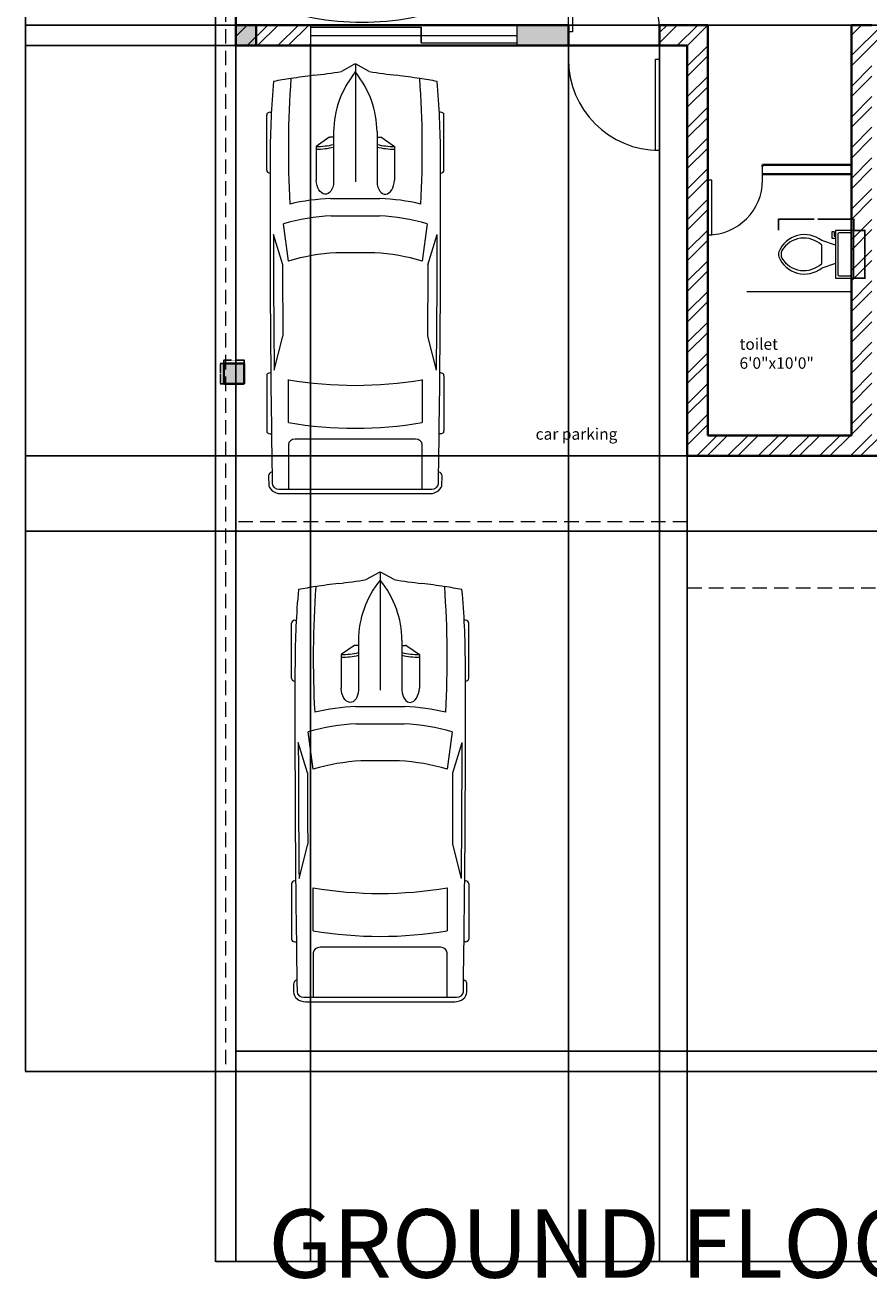
# Model space of a CAD drawing. Units: inches. Extents: x 19613 to 21413, y 12082 to 13202.
# Tile 1 of 9: x 19613 to 19983, y 12084 to 12634. Entities that reach past the tile are written whole.
import ezdxf

# ---------------------------------------------------------------- set-up
doc = ezdxf.new("R2010")
doc.units = ezdxf.units.IN
doc.linetypes.add('HIDDEN', pattern=[9.525, 6.35, -3.175])
for name, color, linetype, lineweight in [('A-ANNO-DIMS', 2, 'Continuous', 18), ('A-ANNO-TEXT', 7, 'Continuous', 30), ('A-AREA-IDEN', 7, 'Continuous', 18), ('A-COLS', 7, 'Continuous', 40), ('A-COLS-PATT', 6, 'Continuous', 13), ('A-DOOR', 3, 'Continuous', 18), ('A-FLOR-FIXT', 9, 'Continuous', 18), ('A-FLOR-HIDN', 8, 'HIDDEN', 13), ('A-FURN', 8, 'Continuous', 18), ('A-GLAZ', 4, 'Continuous', 18), ('A-WALL', 7, 'Continuous', 35), ('A-WALL-PATT', 252, 'Continuous', 13), ('C-PKNG-VEHI', 8, 'Continuous', 13), ('C-PROP', 7, 'Continuous', 25), ('C-PROP-HIDN', 8, 'HIDDEN', 13)]:
    doc.layers.add(name, color=color, linetype=linetype, lineweight=lineweight)
doc.styles.get("Standard").update_dxf_attribs({"font": 'arial.ttf'})
doc.dimstyles.get("Standard").update_dxf_attribs({"dimtxt": 0.18, "dimasz": 0.18, "dimexe": 0.18, "dimexo": 0.0625, "dimgap": 0.09, "dimtad": 0, "dimtih": 1, "dimtoh": 1, "dimdec": 4, "dimzin": 0, "dimdsep": 46, "dimtxsty": 'Standard', "dimcen": 0.09, "dimadec": 0, "dimazin": 0, "dimtfac": 1, "dimtdec": 4, "dimtofl": 0, "dimtmove": 0, "dimatfit": 3, "dimfxl": 1, "dimtolj": 1, "dimtzin": 0, "dimarcsym": 0})

# ---------------------------------------------------------------- blocks, each defined once
blk = doc.blocks.new('*U6')
for p, q in [((0, 0), (0, -6)), ((40, 0), (40, -6))]:
    blk.add_line(p, q)
blk.add_lwpolyline([(0, 0), (0, 40), (1.75, 40), (1.75, 0)], close=True)
blk.add_arc((0, 0), 40, 0, 90)
blk = doc.blocks.new('*U7')
for p, q in [((-40, 0), (-40, 6)), ((0, 0), (0, 6))]:
    blk.add_line(p, q)
blk.add_lwpolyline([(0, 0), (0, -40), (-1.75, -40), (-1.75, 0)], close=True)
blk.add_arc((0, 0), 40, 180, 270)
blk = doc.blocks.new('Sofa - Roundback 7 ft.')
for p, q in [((-12.00002, -32.4421), (-12.00003, -6.5971)), ((11.99997, -32.4421), (11.99998, -6.5971)), ((-36.000027, -34), (-36.000027, -11.4696)), ((-35.999844, -13.3819), (35.9998, -13.3819)), ((35.99998, -34), (35.99998, -11.4696)), ((-36.000027, -32.4421), (35.99998, -32.4421))]:
    blk.add_line(p, q)
for points in [[(-36.000027, -34), (-42.000027, -34), (-42.000027, -8)], [(41.99998, -8), (41.99998, -34), (35.99998, -34)]]:
    blk.add_lwpolyline(points)
for centre, radius, start, end in [((0, -114.25), 114.25, 68.43141, 111.5686), ((-0.00001, -127.1968), 121.1968, 72.72033, 107.2797)]:
    blk.add_arc(centre, radius, start, end)
blk = doc.blocks.new('*U18')
for p, q in [((46.55, 38.89), (22.35, 38.89)), ((136.7, 38.89), (160.9, 38.89)), ((21.1, 37.41), (21.1, 36.83)), ((47.8, 37.39), (47.8, 37.41)), ((87.99, 31.87), (74.76, 35.92)), ((134.31, 35.6), (119.29, 31.78)), ((135.45, 37.07), (135.45, 37.41)), ((162.15, 37.41), (162.15, 36.77)), ((186.47, -33.5), (186.47, 33.5)), ((70.03, 31.54), (86.41, 29.35)), ((138.42, 29.35), (157.25, 29.35)), ((186.47, 29.35), (167.01, 29.35)), ((188.4, -32.76), (188.4, 32.76)), ((164.52, 26.39), (164.52, -26.39)), ((32.27, 11.63), (36.13, 17.17)), ((36.13, 17.17), (50.94, 17.17)), ((32.12, 9.51), (32.12, 11.15)), ((3.27, 6.13), (0.1, 0.41)), ((29.77, 9.51), (51.68, 9.51)), ((58.92, -10.77), (58.92, 10.77)), ((66.55, -10.53), (66.55, 10.53)), ((82.74, 8.5), (82.74, -8.5)), ((186.47, -10.53), (186.47, 10.53)), ((0, 0), (51.68, 0)), ((0.1, -0.41), (3.27, -6.13)), ((29.77, -9.51), (51.68, -9.51)), ((32.12, -9.51), (32.12, -11.15)), ((32.27, -11.63), (36.13, -17.17)), ((36.13, -17.17), (50.94, -17.17)), ((86.41, -29.35), (70.03, -31.54)), ((87.99, -31.87), (74.76, -35.92)), ((134.31, -35.6), (119.29, -31.78)), ((157.25, -29.35), (138.42, -29.35)), ((167.01, -29.35), (186.47, -29.35)), ((21.1, -37.41), (21.1, -36.83)), ((47.8, -37.39), (47.8, -37.41)), ((135.45, -37.07), (135.45, -37.41)), ((162.15, -37.41), (162.15, -36.77)), ((46.55, -38.89), (22.35, -38.89)), ((136.7, -38.89), (160.9, -38.89))]:
    blk.add_line(p, q)
for centre, major_axis, ratio, start_param, end_param in [((22.35, 37.41), (0, -1.48), 0.842304, 3.141593, 4.712389), ((46.55, 37.41), (0, 1.48), 0.842304, -1.570796, 0), ((136.7, 37.41), (0, -1.48), 0.842304, 3.141593, 4.712389), ((160.9, 37.41), (0, 1.48), 0.842304, -1.570796, 0), ((266.03, -27.52), (0, 313.31), 0.842304, 1.367076, 1.39176), ((41.19, -490.86), (0, 528.23), 0.842304, 0.00281, 0.075598), ((64.48, -10555.62), (0, 10593.03), 0.842304, -0.013397, 0.002797), ((64.48, -10555.62), (0, -10591.55), 0.842304, 3.133765, 3.140441), ((180.63, 35.84), (0, 2.22), 0.842304, -0.013017, 1.249894), ((64.48, -10556.36), (0, 10595.31), 0.842304, -0.013397, -0.013017), ((183.98, 33.5), (0, -2.96), 0.842304, 1.570796, 3.128196), ((183.98, 32.76), (0, -5.25), 0.842304, 1.570796, 3.128196), ((259.18, -27.52), (0, -305.3), 0.842304, 4.528606, 4.561838), ((37.47, -593.96), (0, -623.33), 0.842304, 3.096046, 3.200911), ((134.4, 5.39), (0, -89.78), 0.842304, 4.449482, 4.652344), ((135.29, 5.39), (0, 81.77), 0.842304, 1.245306, 1.50788), ((149.6, 2.8), (0, -79.58), 0.842304, 4.372215, 4.640744), ((95.79, -3666.35), (0, -3698.24), 0.842304, 3.134049, 3.144098), ((17.08, 0), (0, 147.02), 0.842304, 4.511394, 4.913384), ((35.91, 0), (0, 147.02), 0.842304, 4.511394, 4.913384), ((167.01, 26.39), (0, 2.96), 0.842304, 0, 1.570796), ((-204.49, 52.4), (0, -250.96), 0.842304, 1.385369, 1.434372), ((13.04, 17.01), (0, 27.42), 0.842304, 4.435146, 4.718221), ((14.2, 17.01), (0, 27.42), 0.842304, 4.435146, 4.718221), ((50.79, 13.34), (6.34, -0.36), 0.603834, -1.395552, 1.581315), ((32.75, 11.15), (0, 0.74), 0.842304, 0.879714, 1.570796), ((29.77, -46.66), (0, 56.17), 0.842304, 0, 0.590319), ((0.62, 0), (0, -0.74), 0.842304, 4.131459, 5.293319), ((29.77, 46.66), (0, 56.17), 0.842304, 2.551274, 3.141593), ((-204.49, -52.4), (0, 250.96), 0.842304, -1.434372, -1.385369), ((13.04, -17.01), (0, -27.42), 0.842304, 1.564964, 1.848039), ((14.2, -17.01), (0, -27.42), 0.842304, 1.564964, 1.848039), ((134.4, -5.39), (0, -89.78), 0.842304, -1.510751, -1.307889), ((135.29, -5.39), (0, -81.77), 0.842304, -1.50788, -1.245306), ((149.6, -2.8), (0, -79.58), 0.842304, -1.499151, -1.230623), ((32.75, -11.15), (0, -0.74), 0.842304, 4.712389, 5.403472), ((259.18, 27.52), (0, 305.3), 0.842304, 1.721348, 1.754579), ((167.01, -26.39), (0, -2.96), 0.842304, 4.712389, 6.283185), ((266.03, 27.52), (0, 313.31), 0.842304, 1.749832, 1.774517), ((37.47, 593.96), (0, -623.33), 0.842304, -0.059319, 0.045547), ((95.79, 3666.35), (0, -3698.24), 0.842304, -0.002505, 0.007544), ((183.98, -32.76), (0, -5.25), 0.842304, 0.013397, 1.570796), ((41.19, 490.86), (0, -528.23), 0.842304, -0.075598, -0.00281), ((22.35, -37.41), (0, 1.48), 0.842304, 1.570796, 3.141593), ((64.48, 10555.62), (0, 10593.03), 0.842304, 3.138796, 3.15499), ((46.55, -37.41), (0, -1.48), 0.842304, 0, 1.570796), ((64.48, 10555.62), (0, -10591.55), 0.842304, 0.001152, 0.007828), ((136.7, -37.41), (0, -1.48), 0.842304, -1.570796, 0), ((160.9, -37.41), (0, 1.48), 0.842304, 3.141593, 4.712389), ((180.63, -35.84), (0, -2.22), 0.842304, -1.249894, 0.013017), ((64.48, 10556.36), (0, 10595.31), 0.842304, 3.15461, 3.15499), ((183.98, -33.5), (0, 2.96), 0.842304, 3.15499, 4.712389)]:
    blk.add_ellipse(centre, major_axis=major_axis, ratio=ratio, start_param=start_param, end_param=end_param)
at = {"extrusion": (0, 0, -1)}
blk.add_ellipse((50.79, -13.34), major_axis=(6.34, 0.36), ratio=0.603834, start_param=-1.395552, end_param=1.581315, dxfattribs=at)
blk = doc.blocks.new('*U19')
for p, q in [((0, 0), (0, 6)), ((24, 0), (24, 6))]:
    blk.add_line(p, q)
blk.add_lwpolyline([(0, 0), (0, -24), (1.75, -24), (1.75, 0)], close=True)
blk.add_arc((0, 0), 24, 270, 0)
blk = doc.blocks.new('Toilet - top')
for p, q in [((9.5, -6), (9.5, -2)), ((-10, -8.5), (-8, -8.5)), ((-10, -9.5), (-10, -8.5)), ((-7, -9.5), (-10, -9.5)), ((-8, -8.5), (-8, -8)), ((-7, -8), (-7, -9.5)), ((-4, -8), (-6, -14)), ((4, -8), (6, -14)), ((4, -14), (-4, -14))]:
    blk.add_line(p, q)
blk.add_lwpolyline([(10.5, -8), (10.5, 0), (-10.5, 0), (-10.5, -8)], close=True)
for points in [[(-9.5, -2), (-9.5, -6)], [(8.5, -1), (-8.5, -1)], [(-8.5, -7), (8.5, -7)]]:
    blk.add_lwpolyline(points)
for centre, radius, start, end in [((-8.62, -1.88), 0.884, 81.8699, 188.1301), ((8.62, -1.88), 0.884, 351.8699, 98.1301), ((-8.62, -6.12), 0.884, 171.8699, 278.1301), ((8.62, -6.12), 0.884, 261.8699, 8.1301), ((3.52, -21.58), 12.17, 141.4691, 247.9714), ((4.2, -21.82), 11.33, 136.3677, 238.9468), ((-3.52, -21.58), 12.17, 292.0284, 38.5307), ((-4.2, -21.82), 11.33, 301.053, 43.6321), ((0, -27.88), 4, 245.7318, 294.2682), ((0, -29), 4, 254.8605, 285.1395)]:
    blk.add_arc(centre, radius, start, end)
blk = doc.blocks.new('COL-9x9')
for p, q in [((0, 9), (9, 9)), ((0, 0), (0, 9)), ((9, 9), (9, 0)), ((9, 0), (0, 0))]:
    blk.add_line(p, q)
blk = doc.blocks.new('WINDOW-LIVING-SLIDER')
for p, q in [((0, 9), (0, 0)), ((0, 8.08), (48.53, 8.08)), ((48.53, 4.5), (48.53, 8.08)), ((48.53, 8.08), (48.53, 1.28)), ((90.49, 9), (90.49, 0)), ((90.49, 6.86), (90.49, 4.5)), ((0, 4.5), (48.53, 4.5)), ((48.53, 1.28), (48.53, 4.5)), ((48.53, 4.5), (90.49, 4.5)), ((48.53, 1.28), (90.49, 1.28))]:
    blk.add_line(p, q)
blk = doc.blocks.new('*D37')
at = {"layer": 'A-ANNO-DIMS', "color": 0, "lineweight": -2, "transparency": 16777216}
for p, q in [((19700.35, 12485.95), (19700.35, 12487.42)), ((19700.53, 12487.24), (19703.81, 12487.24)), ((19709.17, 12487.24), (19705.88, 12487.24)), ((19709.35, 12485.95), (19709.35, 12487.42))]:
    blk.add_line(p, q, dxfattribs=at)
at = {"layer": 'A-ANNO-DIMS', "color": 0, "transparency": 16777216}
for points in [[(19700.53, 12487.27), (19700.53, 12487.21), (19700.35, 12487.24)], [(19709.17, 12487.27), (19709.17, 12487.21), (19709.35, 12487.24)]]:
    blk.add_solid(points, dxfattribs=at)
at = {"layer": 'Defpoints', "color": 0, "transparency": 16777216}
for p in [(19700.35, 12487.24), (19700.35, 12485.89), (19709.35, 12485.89)]:
    blk.add_point(p, dxfattribs=at)
at = {"layer": 'A-ANNO-DIMS', "color": 0, "transparency": 16777216, "insert": (19704.85, 12487.24), "char_height": 0.18, "attachment_point": 5}
blk.add_mtext('\\A1;COLUMN 9 TYP.', dxfattribs=at)
blk = doc.blocks.new('*D38')
at = {"layer": 'A-ANNO-DIMS', "color": 0, "lineweight": -2, "transparency": 16777216}
for p, q in [((19700.29, 12485.89), (19698.82, 12485.89)), ((19699, 12485.71), (19699, 12481.57)), ((19699, 12477.07), (19699, 12481.21)), ((19700.29, 12476.89), (19698.82, 12476.89))]:
    blk.add_line(p, q, dxfattribs=at)
at = {"layer": 'A-ANNO-DIMS', "color": 0, "transparency": 16777216}
for points in [[(19698.97, 12485.71), (19699.03, 12485.71), (19699, 12485.89)], [(19698.97, 12477.07), (19699.03, 12477.07), (19699, 12476.89)]]:
    blk.add_solid(points, dxfattribs=at)
at = {"layer": 'Defpoints', "color": 0, "transparency": 16777216}
for p in [(19700.35, 12485.89), (19699, 12476.89), (19700.35, 12476.89)]:
    blk.add_point(p, dxfattribs=at)
at = {"layer": 'A-ANNO-DIMS', "color": 0, "transparency": 16777216, "insert": (19699, 12481.39), "char_height": 0.18, "attachment_point": 5}
blk.add_mtext('\\A1;9 TYP.', dxfattribs=at)
blk = doc.blocks.new('*D43')
at = {"layer": 'A-ANNO-DIMS', "color": 0, "lineweight": -2, "transparency": 16777216}
for p, q in [((19943.64, 12544.28), (19943.64, 12549.36)), ((19943.82, 12549.18), (19959.39, 12549.18)), ((19976.5, 12549.18), (19960.94, 12549.18)), ((19976.68, 12544.28), (19976.68, 12549.36))]:
    blk.add_line(p, q, dxfattribs=at)
at = {"layer": 'A-ANNO-DIMS', "color": 0, "transparency": 16777216}
for points in [[(19943.82, 12549.21), (19943.82, 12549.15), (19943.64, 12549.18)], [(19976.5, 12549.21), (19976.5, 12549.15), (19976.68, 12549.18)]]:
    blk.add_solid(points, dxfattribs=at)
at = {"layer": 'Defpoints', "color": 0, "transparency": 16777216}
for p in [(19976.68, 12549.18), (19943.64, 12544.22), (19976.68, 12544.22)]:
    blk.add_point(p, dxfattribs=at)
at = {"layer": 'A-ANNO-DIMS', "color": 0, "transparency": 16777216, "insert": (19960.16, 12549.18), "char_height": 0.18, "attachment_point": 5}
blk.add_mtext('\\A1;WC 33 TYP.', dxfattribs=at)
blk = doc.blocks.new('*D44')
at = {"layer": 'A-ANNO-DIMS', "color": 0, "lineweight": -2, "transparency": 16777216}
for p, q in [((19976.75, 12544.22), (19981.82, 12544.22)), ((19981.64, 12544.04), (19981.64, 12533.9)), ((19981.64, 12523.4), (19981.64, 12533.54)), ((19976.75, 12523.22), (19981.82, 12523.22))]:
    blk.add_line(p, q, dxfattribs=at)
at = {"layer": 'A-ANNO-DIMS', "color": 0, "transparency": 16777216}
for points in [[(19981.61, 12544.04), (19981.67, 12544.04), (19981.64, 12544.22)], [(19981.61, 12523.4), (19981.67, 12523.4), (19981.64, 12523.22)]]:
    blk.add_solid(points, dxfattribs=at)
at = {"layer": 'Defpoints', "color": 0, "transparency": 16777216}
for p in [(19976.68, 12544.22), (19976.68, 12523.22), (19981.64, 12523.22)]:
    blk.add_point(p, dxfattribs=at)
at = {"layer": 'A-ANNO-DIMS', "color": 0, "transparency": 16777216, "insert": (19981.64, 12533.72), "char_height": 0.18, "attachment_point": 5}
blk.add_mtext('\\A1;21 TYP.', dxfattribs=at)
blk = doc.blocks.new('*D83')
at = {"layer": 'A-ANNO-DIMS', "color": 0, "lineweight": -2, "transparency": 16777216}
for p, q in [((19696.69, 12175.22), (19696.69, 12091.85)), ((20227.69, 12175.22), (20227.69, 12091.85)), ((19696.87, 12092.03), (19961.92, 12092.03)), ((20227.51, 12092.03), (19962.47, 12092.03))]:
    blk.add_line(p, q, dxfattribs=at)
at = {"layer": 'A-ANNO-DIMS', "color": 0, "transparency": 16777216}
for points in [[(19696.87, 12092.06), (19696.87, 12092), (19696.69, 12092.03)], [(20227.51, 12092.06), (20227.51, 12092), (20227.69, 12092.03)]]:
    blk.add_solid(points, dxfattribs=at)
at = {"layer": 'Defpoints', "color": 0, "transparency": 16777216}
for p in [(19696.69, 12175.28), (20227.69, 12175.28), (20227.69, 12092.03)]:
    blk.add_point(p, dxfattribs=at)
at = {"layer": 'A-ANNO-DIMS', "color": 0, "transparency": 16777216, "insert": (19962.19, 12092.03), "char_height": 0.18, "attachment_point": 5}
blk.add_mtext('\\A1;531', dxfattribs=at)
blk = doc.blocks.new('*D84')
at = {"layer": 'A-ANNO-DIMS', "color": 0, "lineweight": -2, "transparency": 16777216}
for p, q in [((19696.63, 13118.28), (19613.26, 13118.28)), ((19613.44, 13118.1), (19613.44, 12646.96)), ((19613.44, 12175.46), (19613.44, 12646.6)), ((19696.63, 12175.28), (19613.26, 12175.28))]:
    blk.add_line(p, q, dxfattribs=at)
at = {"layer": 'A-ANNO-DIMS', "color": 0, "transparency": 16777216}
for points in [[(19613.41, 13118.1), (19613.47, 13118.1), (19613.44, 13118.28)], [(19613.41, 12175.46), (19613.47, 12175.46), (19613.44, 12175.28)]]:
    blk.add_solid(points, dxfattribs=at)
at = {"layer": 'Defpoints', "color": 0, "transparency": 16777216}
for p in [(19613.44, 13118.28), (19696.69, 13118.28), (19696.69, 12175.28)]:
    blk.add_point(p, dxfattribs=at)
at = {"layer": 'A-ANNO-DIMS', "color": 0, "transparency": 16777216, "insert": (19613.44, 12646.78), "char_height": 0.18, "attachment_point": 5}
blk.add_mtext('\\A1;943', dxfattribs=at)
blk = doc.blocks.new('*D89')
at = {"layer": 'A-ANNO-DIMS', "color": 0, "lineweight": -2, "transparency": 16777216}
for p, q in [((20807.37, 12808.28), (19613.26, 12808.28)), ((19613.44, 12808.1), (19613.44, 12721.46)), ((19613.44, 12634.46), (19613.44, 12721.1)), ((20807.37, 12634.28), (19613.26, 12634.28))]:
    blk.add_line(p, q, dxfattribs=at)
at = {"layer": 'A-ANNO-DIMS', "color": 0, "transparency": 16777216}
for points in [[(19613.41, 12808.1), (19613.47, 12808.1), (19613.44, 12808.28)], [(19613.41, 12634.46), (19613.47, 12634.46), (19613.44, 12634.28)]]:
    blk.add_solid(points, dxfattribs=at)
at = {"layer": 'Defpoints', "color": 0, "transparency": 16777216}
for p in [(19613.44, 12808.28), (20807.43, 12808.28), (20807.43, 12634.28)]:
    blk.add_point(p, dxfattribs=at)
at = {"layer": 'A-ANNO-DIMS', "color": 0, "transparency": 16777216, "insert": (19613.44, 12721.28), "char_height": 0.18, "attachment_point": 5}
blk.add_mtext('\\A1;174', dxfattribs=at)
blk = doc.blocks.new('*D91')
at = {"layer": 'A-ANNO-DIMS', "color": 0, "lineweight": -2, "transparency": 16777216}
for p, q in [((19851.55, 12625.22), (19851.55, 12091.85)), ((19891.55, 12625.22), (19891.55, 12091.85)), ((19851.73, 12092.03), (19871.33, 12092.03)), ((19891.37, 12092.03), (19871.77, 12092.03))]:
    blk.add_line(p, q, dxfattribs=at)
at = {"layer": 'A-ANNO-DIMS', "color": 0, "transparency": 16777216}
for points in [[(19851.73, 12092.06), (19851.73, 12092), (19851.55, 12092.03)], [(19891.37, 12092.06), (19891.37, 12092), (19891.55, 12092.03)]]:
    blk.add_solid(points, dxfattribs=at)
at = {"layer": 'Defpoints', "color": 0, "transparency": 16777216}
for p in [(19851.55, 12625.28), (19891.55, 12625.28), (19891.55, 12092.03)]:
    blk.add_point(p, dxfattribs=at)
at = {"layer": 'A-ANNO-DIMS', "color": 0, "transparency": 16777216, "insert": (19871.55, 12092.03), "char_height": 0.18, "attachment_point": 5}
blk.add_mtext('\\A1;40', dxfattribs=at)
blk = doc.blocks.new('*D92')
at = {"layer": 'A-ANNO-DIMS', "color": 0, "lineweight": -2, "transparency": 16777216}
for p, q in [((19903.69, 12445.22), (19903.69, 12091.85)), ((20128.69, 12445.22), (20128.69, 12091.85)), ((19903.87, 12092.03), (20015.9, 12092.03)), ((20128.51, 12092.03), (20016.48, 12092.03))]:
    blk.add_line(p, q, dxfattribs=at)
at = {"layer": 'A-ANNO-DIMS', "color": 0, "transparency": 16777216}
for points in [[(19903.87, 12092.06), (19903.87, 12092), (19903.69, 12092.03)], [(20128.51, 12092.06), (20128.51, 12092), (20128.69, 12092.03)]]:
    blk.add_solid(points, dxfattribs=at)
at = {"layer": 'Defpoints', "color": 0, "transparency": 16777216}
for p in [(19903.69, 12445.28), (20128.69, 12445.28), (20128.69, 12092.03)]:
    blk.add_point(p, dxfattribs=at)
at = {"layer": 'A-ANNO-DIMS', "color": 0, "transparency": 16777216, "insert": (20016.19, 12092.03), "char_height": 0.18, "attachment_point": 5}
blk.add_mtext('\\A1;225', dxfattribs=at)
blk = doc.blocks.new('*D96')
at = {"layer": 'A-ANNO-DIMS', "color": 0, "lineweight": -2, "transparency": 16777216}
for p, q in [((19903.63, 12625.28), (19613.26, 12625.28)), ((19613.44, 12625.1), (19613.44, 12535.46)), ((19613.44, 12445.46), (19613.44, 12535.1)), ((19903.63, 12445.28), (19613.26, 12445.28))]:
    blk.add_line(p, q, dxfattribs=at)
at = {"layer": 'A-ANNO-DIMS', "color": 0, "transparency": 16777216}
for points in [[(19613.41, 12625.1), (19613.47, 12625.1), (19613.44, 12625.28)], [(19613.41, 12445.46), (19613.47, 12445.46), (19613.44, 12445.28)]]:
    blk.add_solid(points, dxfattribs=at)
at = {"layer": 'Defpoints', "color": 0, "transparency": 16777216}
for p in [(19613.44, 12625.28), (19903.69, 12625.28), (19903.69, 12445.28)]:
    blk.add_point(p, dxfattribs=at)
at = {"layer": 'A-ANNO-DIMS', "color": 0, "transparency": 16777216, "insert": (19613.44, 12535.28), "char_height": 0.18, "attachment_point": 5}
blk.add_mtext('\\A1;180', dxfattribs=at)
blk = doc.blocks.new('*D97')
at = {"layer": 'A-ANNO-DIMS', "color": 0, "lineweight": -2, "transparency": 16777216}
for p, q in [((20128.63, 12445.28), (19613.26, 12445.28)), ((19613.44, 12445.1), (19613.44, 12428.96)), ((19613.44, 12412.46), (19613.44, 12428.6)), ((20128.63, 12412.28), (19613.26, 12412.28))]:
    blk.add_line(p, q, dxfattribs=at)
at = {"layer": 'A-ANNO-DIMS', "color": 0, "transparency": 16777216}
for points in [[(19613.41, 12445.1), (19613.47, 12445.1), (19613.44, 12445.28)], [(19613.41, 12412.46), (19613.47, 12412.46), (19613.44, 12412.28)]]:
    blk.add_solid(points, dxfattribs=at)
at = {"layer": 'Defpoints', "color": 0, "transparency": 16777216}
for p in [(19613.44, 12445.28), (20128.69, 12445.28), (20128.69, 12412.28)]:
    blk.add_point(p, dxfattribs=at)
at = {"layer": 'A-ANNO-DIMS', "color": 0, "transparency": 16777216, "insert": (19613.44, 12428.78), "char_height": 0.18, "attachment_point": 5}
blk.add_mtext('\\A1;33', dxfattribs=at)
blk = doc.blocks.new('*D105')
at = {"layer": 'A-ANNO-DIMS', "color": 0, "lineweight": -2, "transparency": 16777216}
for p, q in [((19705.69, 12625.22), (19705.69, 12091.85)), ((19738.39, 12625.22), (19738.39, 12091.85)), ((19705.87, 12092.03), (19721.72, 12092.03)), ((19738.21, 12092.03), (19722.37, 12092.03))]:
    blk.add_line(p, q, dxfattribs=at)
at = {"layer": 'A-ANNO-DIMS', "color": 0, "transparency": 16777216}
for points in [[(19705.87, 12092.06), (19705.87, 12092), (19705.69, 12092.03)], [(19738.21, 12092.06), (19738.21, 12092), (19738.39, 12092.03)]]:
    blk.add_solid(points, dxfattribs=at)
at = {"layer": 'Defpoints', "color": 0, "transparency": 16777216}
for p in [(19705.69, 12625.28), (19738.39, 12625.28), (19738.39, 12092.03)]:
    blk.add_point(p, dxfattribs=at)
at = {"layer": 'A-ANNO-DIMS', "color": 0, "transparency": 16777216, "insert": (19722.04, 12092.03), "char_height": 0.18, "attachment_point": 5}
blk.add_mtext('\\A1;32.7', dxfattribs=at)
blk = doc.blocks.new('*D106')
at = {"layer": 'A-ANNO-DIMS', "color": 0, "lineweight": -2, "transparency": 16777216}
for p, q in [((19891.55, 12625.22), (19891.55, 12091.85)), ((19903.69, 12625.22), (19903.69, 12091.85)), ((19891.73, 12092.03), (19897.17, 12092.03)), ((19903.51, 12092.03), (19898.08, 12092.03))]:
    blk.add_line(p, q, dxfattribs=at)
at = {"layer": 'A-ANNO-DIMS', "color": 0, "transparency": 16777216}
for points in [[(19891.73, 12092.06), (19891.73, 12092), (19891.55, 12092.03)], [(19903.51, 12092.06), (19903.51, 12092), (19903.69, 12092.03)]]:
    blk.add_solid(points, dxfattribs=at)
at = {"layer": 'Defpoints', "color": 0, "transparency": 16777216}
for p in [(19891.55, 12625.28), (19903.69, 12625.28), (19903.69, 12092.03)]:
    blk.add_point(p, dxfattribs=at)
at = {"layer": 'A-ANNO-DIMS', "color": 0, "transparency": 16777216, "insert": (19897.62, 12092.03), "char_height": 0.18, "attachment_point": 5}
blk.add_mtext('\\A1;12.143', dxfattribs=at)

msp = doc.modelspace()

# ---------------------------------------------------------------- hatches: boundary and pattern name
at = {"layer": 'A-COLS-PATT'}
h = msp.add_hatch(color=256, dxfattribs=at)
h.dxf.hatch_style = 1
h.paths.add_polyline_path([(19701.1937, 13118.279), (19696.6937, 13118.279), (19696.6937, 13113.779), (19701.1937, 13113.779)])
h.paths.add_polyline_path([(19714.6694, 12982.279), (19705.6937, 12982.279), (19705.6937, 12973.279), (19714.6694, 12973.279)])
h.paths.add_polyline_path([(19827.1183, 12982.279), (19818.1183, 12982.279), (19818.1183, 12973.279), (19827.1183, 12973.279)])
h.paths.add_polyline_path([(19982.6937, 12982.279), (19973.6937, 12982.279), (19973.6937, 12973.279), (19982.6937, 12973.279)])
h.paths.add_polyline_path([(19982.6937, 12817.279), (19973.6937, 12817.279), (19973.6937, 12808.279), (19982.6937, 12808.279)])
h.paths.add_polyline_path([(19795.361, 12817.279), (19786.361, 12817.279), (19786.361, 12808.279), (19795.361, 12808.279)])
h.paths.add_polyline_path([(19705.6937, 12817.279), (19702.0819, 12817.279), (19702.0819, 12808.279), (19705.6937, 12808.279)])
h.paths.add_polyline_path([(19711.0819, 12817.279), (19705.6937, 12817.279), (19705.6937, 12808.279), (19711.0819, 12808.279)])
h.paths.add_polyline_path([(19714.6136, 12634.279), (19705.6937, 12634.279), (19705.6937, 12625.279), (19714.6136, 12625.279)])
h.paths.add_polyline_path([(19705.6937, 12485.8897), (19701.1937, 12485.8897), (19701.1937, 12476.8897), (19705.6937, 12476.8897)])
h.paths.add_polyline_path([(19709.3479, 12485.8897), (19705.6937, 12485.8897), (19705.6937, 12476.8897), (19709.3479, 12476.8897)])
h.paths.add_polyline_path([(19701.1937, 12485.8897), (19700.3479, 12485.8897), (19700.3479, 12476.8897), (19701.1937, 12476.8897)])
h.paths.add_polyline_path([(20218.6937, 12421.279), (20209.6937, 12421.279), (20209.6937, 12412.279), (20218.6937, 12412.279)])
h.paths.add_polyline_path([(20218.6937, 12634.279), (20209.6937, 12634.279), (20209.6937, 12625.279), (20218.6937, 12625.279)])
h.paths.add_polyline_path([(20218.6937, 12808.279), (20209.6937, 12808.279), (20209.6937, 12803.279), (20218.6937, 12803.279)])
h.paths.add_polyline_path([(20218.6937, 12810.1878), (20209.6937, 12810.1878), (20209.6937, 12808.279), (20218.6937, 12808.279)])
h.paths.add_polyline_path([(20218.6937, 12803.279), (20209.6937, 12803.279), (20209.6937, 12801.1878), (20218.6937, 12801.1878)])
h.paths.add_polyline_path([(20218.6937, 12982.279), (20209.6937, 12982.279), (20209.6937, 12973.279), (20218.6937, 12973.279)])
h.paths.add_polyline_path([(20100.1214, 12982.279), (20080.8386, 12982.279), (20080.8386, 12973.279), (20091.6937, 12973.279), (20100.1214, 12973.279), (20100.1214, 12976.279)])
h.paths.add_polyline_path([(19851.5503, 12631.279), (19851.5503, 12634.279), (19828.8814, 12634.279), (19828.8814, 12625.279), (19851.5503, 12625.279)])
at = {"layer": 'A-WALL-PATT'}
h = msp.add_hatch(dxfattribs=at)
h.set_pattern_fill('ANSI32', color=256)
h.paths.add_polyline_path([(20223.1937, 13118.279), (20218.6937, 13118.279), (19701.1937, 13118.279), (19701.1937, 13113.779), (20223.1937, 13113.779)])
h.paths.add_polyline_path([(19849.7315, 12982.279), (19799.9854, 12982.279), (19799.9854, 12973.279), (19849.7315, 12973.279)])
h.paths.add_polyline_path([(19755.5378, 12982.279), (19705.6937, 12982.279), (19705.6937, 12973.279), (19755.5378, 12973.279)])
h.paths.add_polyline_path([(20000.1054, 12982.279), (19950.0534, 12982.279), (19950.0534, 12974.1171), (19950.0534, 12973.279), (20000.1054, 12973.279)])
h.paths.add_polyline_path([(20049.4797, 12982.279), (20030.7476, 12982.279), (20030.7476, 12973.279), (20049.4797, 12973.279)])
h.paths.add_polyline_path([(20100.1214, 12982.279), (20080.8386, 12982.279), (20080.8386, 12973.279), (20100.1214, 12973.279), (20100.1214, 12976.279)])
h.paths.add_polyline_path([(20218.6937, 12982.279), (20167.6937, 12982.279), (20140.1214, 12982.279), (20140.1214, 12976.279, -0.01769781), (20140.0212, 12973.45), (20167.6937, 12973.279), (20176.6937, 12973.279), (20218.6937, 12973.279)])
h.paths.add_polyline_path([(19851.5503, 12814.279), (19851.5503, 12817.279), (19793.6937, 12817.279), (19789.6937, 12817.279), (19705.6937, 12817.279), (19705.6937, 12808.279), (19851.5503, 12808.279)])
h.paths.add_polyline_path([(19982.6937, 12973.279), (19973.6937, 12973.279), (19973.6937, 12817.279), (19887.5503, 12817.279), (19887.5503, 12808.279), (19973.6937, 12808.279), (19982.6937, 12808.279)])
h.paths.add_polyline_path([(20058.6937, 12850.5529), (19982.6937, 12850.5529), (19982.6937, 12846.5529), (20058.6937, 12846.5529)])
h.paths.add_polyline_path([(20095.6937, 12973.279), (20091.6937, 12973.279), (20091.6937, 12850.5529), (20087.6937, 12850.5529), (20087.6937, 12846.5529), (20095.6937, 12846.5529)])
h.paths.add_polyline_path([(20218.6937, 12808.279), (20140.8605, 12808.279), (20126.9413, 12808.279), (20126.9413, 12803.279), (20140.8605, 12803.279), (20218.6937, 12803.279)])
h.paths.add_polyline_path([(19738.3931, 12634.279), (19705.6937, 12634.279), (19705.6937, 12625.279), (19738.3931, 12625.279)])
h.paths.add_polyline_path([(19912.6937, 12634.279), (19903.6937, 12634.279), (19891.5503, 12634.279), (19891.5503, 12625.279), (19903.6937, 12625.279), (19903.6937, 12445.279), (19975.6937, 12445.279), (20128.6937, 12445.279), (20128.6937, 12412.279), (20149.8479, 12412.279), (20149.8479, 12421.279), (20137.6937, 12421.279), (20137.6937, 12454.279), (20137.6937, 12580.2801), (20133.6937, 12580.2801), (20133.6937, 12454.279), (19984.6937, 12454.279), (19984.6937, 12625.279), (19993.6937, 12625.279), (19993.6937, 12634.279), (19984.6937, 12634.279), (19975.6937, 12634.279), (19975.6937, 12454.279), (19912.6937, 12454.279)])
h.paths.add_polyline_path([(20218.6937, 12634.279), (20137.6937, 12634.279), (20029.6937, 12634.279), (20029.6937, 12625.279), (20137.6937, 12625.279), (20218.6937, 12625.279)])
h.paths.add_polyline_path([(21014.4339, 12634.279), (21005.4339, 12634.279), (20993.2905, 12634.279), (20993.2905, 12625.279), (21005.4339, 12625.279), (21005.4339, 12445.279), (21077.4339, 12445.279), (21230.4339, 12445.279), (21230.4339, 12412.279), (21251.5881, 12412.279), (21251.5881, 12421.279), (21239.4339, 12421.279), (21239.4339, 12454.279), (21239.4339, 12580.2801), (21235.4339, 12580.2801), (21235.4339, 12454.279), (21086.4339, 12454.279), (21086.4339, 12625.279), (21095.4339, 12625.279), (21095.4339, 12634.279), (21086.4339, 12634.279), (21077.4339, 12634.279), (21077.4339, 12454.279), (21014.4339, 12454.279)])
h.paths.add_polyline_path([(20840.1333, 12634.279), (20807.4339, 12634.279), (20807.4339, 12625.279), (20840.1333, 12625.279)])
h.paths.add_polyline_path([(20953.2905, 12631.279), (20953.2905, 12634.279), (20930.6216, 12634.279), (20930.6216, 12625.279), (20953.2905, 12625.279)])
h.paths.add_polyline_path([(21320.4339, 12634.279), (21239.4339, 12634.279), (21131.4339, 12634.279), (21131.4339, 12625.279), (21239.4339, 12625.279), (21320.4339, 12625.279)])
h.paths.add_polyline_path([(21084.4339, 12973.279), (21075.4339, 12973.279), (21075.4339, 12817.279), (20989.2905, 12817.279), (20989.2905, 12808.279), (21075.4339, 12808.279), (21084.4339, 12808.279)])
h.paths.add_polyline_path([(21142.1261, 12863.2893), (21084.4339, 12863.2893), (21084.4339, 12846.5529), (21142.1261, 12846.5529)])
h.paths.add_polyline_path([(21320.4339, 12808.279), (21242.6007, 12808.279), (21228.6815, 12808.279), (21228.6815, 12803.279), (21242.6007, 12803.279), (21320.4339, 12803.279)])
h.paths.add_polyline_path([(20857.278, 12982.279), (20807.4339, 12982.279), (20807.4339, 12973.279), (20857.278, 12973.279)])
h.paths.add_polyline_path([(20951.4717, 12982.279), (20901.7255, 12982.279), (20901.7255, 12973.279), (20951.4717, 12973.279)])
h.paths.add_polyline_path([(21101.8455, 12982.279), (21051.7936, 12982.279), (21051.7936, 12974.1171), (21051.7936, 12973.279), (21101.8455, 12973.279)])
h.paths.add_polyline_path([(21151.2199, 12982.279), (21132.4878, 12982.279), (21132.4878, 12973.279), (21151.2199, 12973.279)])
h.paths.add_polyline_path([(21201.8616, 12982.279), (21182.5788, 12982.279), (21182.5788, 12973.279), (21193.4339, 12973.279), (21201.8616, 12973.279), (21201.8616, 12976.279)])
h.paths.add_polyline_path([(21320.4339, 12982.279), (21269.4339, 12982.279), (21241.8616, 12982.279), (21241.8616, 12976.279, -0.01769781), (21241.7614, 12973.45), (21269.4339, 12973.279), (21278.4339, 12973.279), (21320.4339, 12973.279)])
h.paths.add_polyline_path([(20953.2905, 12817.279), (20895.4339, 12817.279), (20891.4339, 12817.279), (20807.4339, 12817.279), (20807.4339, 12808.279), (20953.2905, 12808.279)])
h.paths.add_polyline_path([(21197.4339, 12973.279), (21193.4339, 12973.279), (21193.4339, 12850.5529), (21197.4339, 12850.5529)])
h.paths.add_polyline_path([(21320.4339, 12550.279), (21272.5278, 12550.279), (21272.5278, 12546.279), (21320.4339, 12546.279)])
h.paths.add_polyline_path([(21320.4339, 12421.279), (21283.2222, 12421.279), (21283.2222, 12412.279), (21320.4339, 12412.279)])

# ---------------------------------------------------------------- linework, layer by layer
at = {"layer": 'A-FLOR-FIXT'}
for p, q in [((19975.6937, 12517.279), (19929.8429, 12517.279)), ((19975.6937, 12454.279), (19975.6937, 12517.279))]:
    msp.add_line(p, q, dxfattribs=at)
at = {"layer": 'A-FLOR-HIDN'}
for p, q in [((19903.6937, 12445.279), (19903.6937, 12387.4793)), ((19903.6937, 12416.3791), (19705.6937, 12416.3791)), ((19903.6937, 12387.4793), (19986.7757, 12387.4793))]:
    msp.add_line(p, q, dxfattribs=at)
at = {"layer": 'A-WALL'}
for p, q in [((19705.6937, 12808.279), (19705.6937, 12634.279)), ((19705.6937, 12634.279), (19851.5503, 12634.279)), ((19705.6937, 12634.279), (19746.4169, 12634.279)), ((19851.5503, 12634.279), (19851.5503, 12625.279)), ((19903.6937, 12634.279), (19891.5503, 12634.279)), ((19891.5503, 12634.279), (19891.5503, 12625.279)), ((19903.6937, 12634.279), (19912.6937, 12634.279)), ((19912.6937, 12454.279), (19912.6937, 12634.279)), ((19975.6937, 12634.279), (19975.6937, 12454.279)), ((19975.6937, 12634.279), (19984.6937, 12634.279)), ((19851.5503, 12625.279), (19705.6937, 12625.279)), ((19851.5503, 12625.279), (19903.6937, 12625.279)), ((19891.5503, 12625.279), (19903.6937, 12625.279)), ((19903.6937, 12445.279), (19903.6937, 12625.279)), ((19975.6937, 12572.9433), (19936.6937, 12572.9433)), ((19936.6937, 12572.2779), (19936.6937, 12572.9433)), ((19936.6937, 12568.9433), (19975.6937, 12568.9433)), ((19975.6937, 12454.279), (19912.6937, 12454.279)), ((19975.6937, 12445.279), (19903.6937, 12445.279)), ((19975.6937, 12445.279), (20128.6937, 12445.279))]:
    msp.add_line(p, q, dxfattribs=at)
at = {"layer": 'C-PROP'}
for p, q in [((19696.6937, 12175.279), (19696.6937, 13118.279)), ((19705.6937, 13109.279), (19705.6937, 12184.279)), ((19696.6937, 12175.279), (19696.6937, 12184.279)), ((19705.6937, 12184.279), (20218.6937, 12184.279)), ((20227.6937, 12175.279), (19696.6937, 12175.279))]:
    msp.add_line(p, q, dxfattribs=at)
at = {"layer": 'C-PROP-HIDN'}
msp.add_line((19701.1937, 13118.279), (19701.1937, 12175.279), dxfattribs=at)

# ---------------------------------------------------------------- block references
at = {"layer": 'A-COLS', "rotation": 180}
for p in [(19714.614, 12634.279), (19709.3483, 12485.8897)]:
    msp.add_blockref('COL-9x9', p, dxfattribs=at)
at = {"layer": 'A-DOOR'}
for name, p in [('*U6', (19851.5503, 12631.279)), ('*U7', (19891.5503, 12619.279)), ('*U19', (19912.6937, 12566.2779))]:
    msp.add_blockref(name, p, dxfattribs=at)
at = {"layer": 'A-FLOR-FIXT', "rotation": 270}
msp.add_blockref('Toilet - top', (19976.6848, 12533.7215), dxfattribs=at)
at = {"layer": 'A-FURN', "rotation": 180}
msp.add_blockref('Sofa - Roundback 7 ft.', (19761.0303, 12635.5266), dxfattribs=at)
at = {"layer": 'A-GLAZ'}
msp.add_blockref('WINDOW-LIVING-SLIDER', (19738.393, 12625.279), dxfattribs=at)
at = {"layer": 'C-PKNG-VEHI', "rotation": 270}
for p in [(19758.0964, 12617.1704), (19769.0083, 12394.309)]:
    msp.add_blockref('*U18', p, dxfattribs=at)

# ---------------------------------------------------------------- texts
at = {"layer": 'A-ANNO-TEXT', "insert": (19719.9437, 12114.8481), "char_height": 30, "attachment_point": 1}
msp.add_mtext_dynamic_manual_height_columns('GROUND FLOOR PLAN', width=510.437427, gutter_width=12.5, heights=[0], dxfattribs=at)
at = {"layer": 'A-AREA-IDEN', "char_height": 5, "attachment_point": 1}
for s, width, insert in [('toilet\\P6\'0"x10\'0"', 19.652904, (19926.601, 12496.8558)), ('car parking', 37.101035, (19837.1733, 12457.4158))]:
    msp.add_mtext_dynamic_manual_height_columns(s, width=width, gutter_width=12.5, heights=[0], dxfattribs=dict(at, insert=insert))

# ---------------------------------------------------------------- dimensions: what is measured, and where the dimension line sits
at = {"layer": 'A-ANNO-DIMS'}
for base, p1, p2, picture, middle in [((19613.4437, 13118.279), (19696.6937, 12175.279), (19696.6937, 13118.279), '*D84', (19613.4437, 12646.779)), ((19613.4437, 12808.279), (20807.4339, 12634.279), (20807.4339, 12808.279), '*D89', (19613.4437, 12721.279)), ((19613.4437, 12625.279), (19903.6937, 12445.279), (19903.6937, 12625.279), '*D96', (19613.4437, 12535.279)), ((19613.4437, 12445.279), (20128.6937, 12412.279), (20128.6937, 12445.279), '*D97', (19613.4437, 12428.779))]:
    dim = msp.add_linear_dim(base=base, p1=p1, p2=p2, angle=90, dimstyle='Standard', override={"dimdec": 0, "dimlfac": 1, "dimrnd": 0, "dimzin": 0, "dimdsep": 46, "dimlunit": 2}, dxfattribs=at)
    dim.commit()
    dim.dimension.update_dxf_attribs({"geometry": picture, "text_midpoint": middle})
for base, p1, p2, override, picture, middle in [((19738.3931, 12092.029), (19705.6937, 12625.279), (19738.3931, 12625.279), {"dimdec": 1, "dimlfac": 1, "dimrnd": 0, "dimzin": 0, "dimdsep": 46, "dimlunit": 2}, '*D105', (19722.0434, 12092.029)), ((19891.5503, 12092.029), (19851.5503, 12625.279), (19891.5503, 12625.279), {"dimdec": 0, "dimlfac": 1, "dimrnd": 0, "dimzin": 0, "dimdsep": 46, "dimlunit": 2}, '*D91', (19871.5503, 12092.029)), ((19903.6937, 12092.029), (19891.5503, 12625.279), (19903.6937, 12625.279), {"dimdec": 3, "dimlfac": 1, "dimrnd": 0, "dimzin": 0, "dimdsep": 46, "dimlunit": 2}, '*D106', (19897.622, 12092.029)), ((20128.6937, 12092.029), (19903.6937, 12445.279), (20128.6937, 12445.279), {"dimdec": 0, "dimlfac": 1, "dimrnd": 0, "dimzin": 0, "dimdsep": 46, "dimlunit": 2}, '*D92', (20016.1937, 12092.029)), ((20227.6937, 12092.029), (19696.6937, 12175.279), (20227.6937, 12175.279), {"dimdec": 0, "dimlfac": 1, "dimrnd": 0, "dimzin": 0, "dimdsep": 46, "dimlunit": 2}, '*D83', (19962.1937, 12092.029))]:
    dim = msp.add_linear_dim(base=base, p1=p1, p2=p2, dimstyle='Standard', override=override, dxfattribs=at)
    dim.commit()
    dim.dimension.update_dxf_attribs({"geometry": picture, "text_midpoint": middle})
dim = msp.add_linear_dim(base=(19976.6848, 12549.1785), p1=(19943.6386, 12544.2215), p2=(19976.6848, 12544.2215), text='WC <> TYP.', dimstyle='Standard', override={"dimdec": 0, "dimlfac": 1, "dimrnd": 0, "dimzin": 0, "dimdsep": 46, "dimlunit": 2}, dxfattribs=at)
dim.commit()
dim.dimension.update_dxf_attribs({"geometry": '*D43', "text_midpoint": (19960.1617, 12549.1785)})
for base, p1, p2, angle, text, picture, middle in [((19981.6418, 12523.2215), (19976.6848, 12544.2215), (19976.6848, 12523.2215), 270, '<> TYP.', '*D44', (19981.6418, 12533.7215)), ((19698.9979, 12476.8897), (19700.3479, 12485.8897), (19700.3479, 12476.8897), 270, '<> TYP.', '*D38', (19698.9979, 12481.3897)), ((19700.3479, 12487.2397), (19709.3479, 12485.8897), (19700.3479, 12485.8897), 180, 'COLUMN <> TYP.', '*D37', (19704.8479, 12487.2397))]:
    dim = msp.add_linear_dim(base=base, p1=p1, p2=p2, angle=angle, text=text, dimstyle='Standard', override={"dimdec": 0, "dimlfac": 1, "dimrnd": 0, "dimzin": 0, "dimdsep": 46, "dimlunit": 2}, dxfattribs=at)
    dim.commit()
    dim.dimension.update_dxf_attribs({"geometry": picture, "text_midpoint": middle})

doc.saveas('drawing.dxf')
